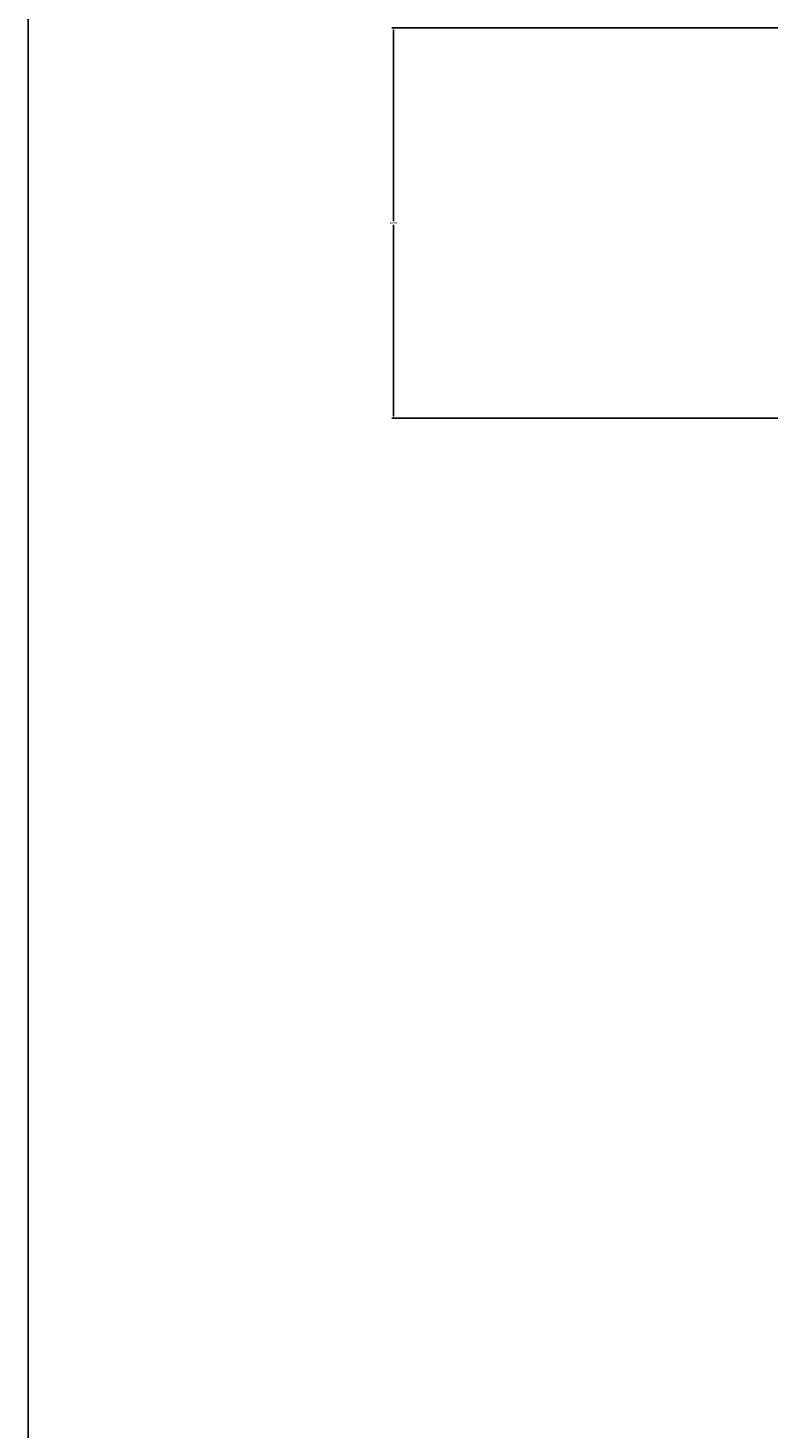
# Model space of a CAD drawing. Units: inches. Extents: x 1601 to 2297, y 1496 to 2631.
# Tile 38 of 57: x 1601 to 1675, y 2391 to 2532. Entities that reach past the tile are written whole.
import ezdxf

# ---------------------------------------------------------------- set-up
doc = ezdxf.new("R2010")
doc.units = ezdxf.units.IN
doc.layers.add('A-ANNO-DIMS', color=2, linetype='Continuous', lineweight=18)
doc.layers.add('A-ANNO-TTLB', color=7, linetype='Continuous', lineweight=25)
doc.styles.get("Standard").update_dxf_attribs({"font": 'arial.ttf'})
doc.dimstyles.get("Standard").update_dxf_attribs({"dimtxt": 0.18, "dimasz": 0.18, "dimexe": 0.18, "dimexo": 0.0625, "dimgap": 0.09, "dimtad": 0, "dimtih": 1, "dimtoh": 1, "dimdec": 4, "dimzin": 0, "dimdsep": 46, "dimtxsty": 'Standard', "dimcen": 0.09, "dimadec": 0, "dimazin": 0, "dimtfac": 1, "dimtdec": 4, "dimtofl": 0, "dimtmove": 0, "dimatfit": 3, "dimfxl": 1, "dimtolj": 1, "dimtzin": 0, "dimarcsym": 0})

# ---------------------------------------------------------------- blocks, each defined once
blk = doc.blocks.new('*D35')
at = {"layer": 'A-ANNO-DIMS', "color": 0, "lineweight": -2, "transparency": 16777216}
for p, q in [((1685.97, 2532.33), (1637.31, 2532.33)), ((1637.49, 2532.15), (1637.49, 2512.82)), ((1637.49, 2493.13), (1637.49, 2512.46)), ((1685.97, 2492.95), (1637.31, 2492.95))]:
    blk.add_line(p, q, dxfattribs=at)
at = {"layer": 'A-ANNO-DIMS', "color": 0, "transparency": 16777216}
for points in [[(1637.46, 2532.15), (1637.52, 2532.15), (1637.49, 2532.33)], [(1637.46, 2493.13), (1637.52, 2493.13), (1637.49, 2492.95)]]:
    blk.add_solid(points, dxfattribs=at)
at = {"layer": 'Defpoints', "color": 0, "transparency": 16777216}
for p in [(1637.49, 2532.33), (1686.04, 2532.33), (1686.04, 2492.95)]:
    blk.add_point(p, dxfattribs=at)
at = {"layer": 'A-ANNO-DIMS', "color": 0, "transparency": 16777216, "insert": (1637.49, 2512.64), "char_height": 0.18, "attachment_point": 5}
blk.add_mtext('\\A1;39.376', dxfattribs=at)

msp = doc.modelspace()

# ---------------------------------------------------------------- linework, layer by layer
at = {"layer": 'A-ANNO-TTLB'}
msp.add_lwpolyline([(1600.5933, 2631.1477), (2297.129, 2631.1477), (2297.129, 1496.1026), (1600.5933, 1496.1026)], close=True, dxfattribs=at)

# ---------------------------------------------------------------- dimensions: what is measured, and where the dimension line sits
at = {"layer": 'A-ANNO-DIMS'}
dim = msp.add_linear_dim(base=(1637.4873, 2532.3254), p1=(1686.0373, 2492.9493), p2=(1686.0373, 2532.3254), angle=90, dimstyle='Standard', override={"dimdec": 3, "dimlfac": 1, "dimrnd": 0, "dimzin": 0, "dimdsep": 46, "dimlunit": 2}, dxfattribs=at)
dim.commit()
dim.dimension.update_dxf_attribs({"geometry": '*D35', "text_midpoint": (1637.4873, 2512.6374)})

doc.saveas('drawing.dxf')
